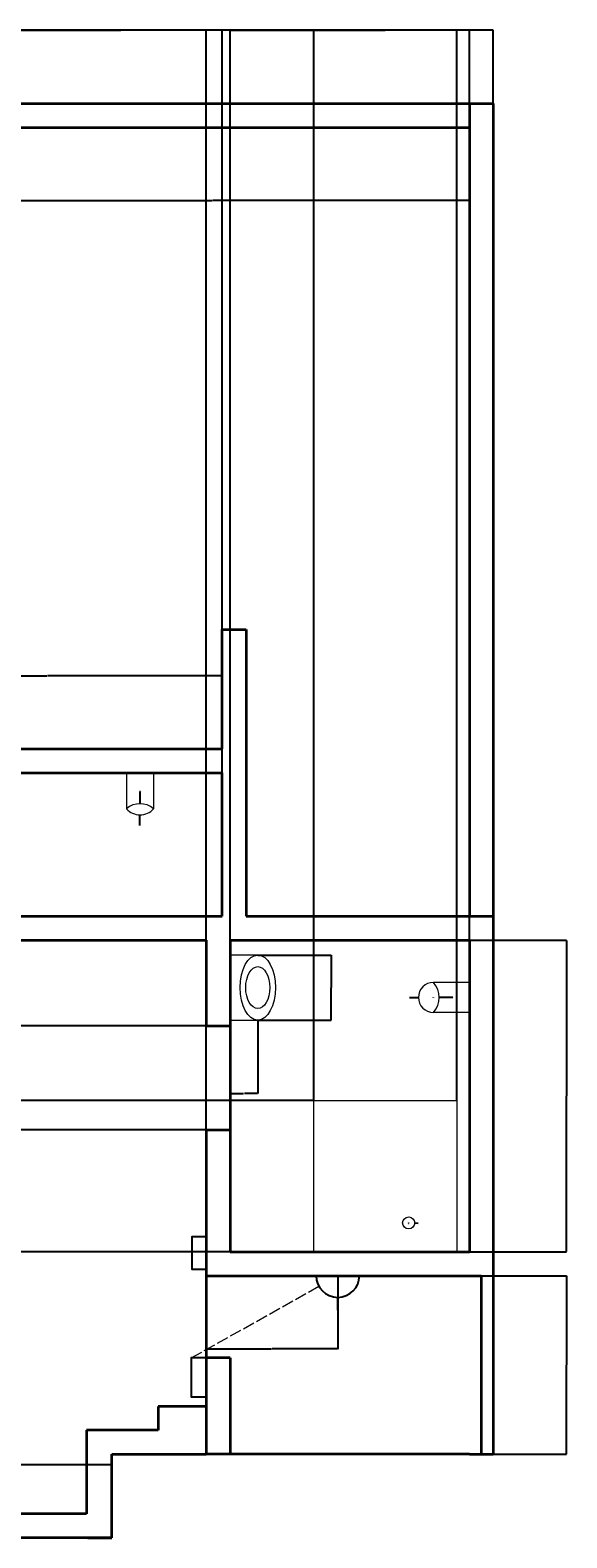
# Model space of a CAD drawing. Units: inches. Extents: x 2034 to 3646, y 962 to 2549.
# Tile 4 of 4: x 3108 to 3646, y 1036 to 2549. Entities that reach past the tile are written whole.
import ezdxf

# ---------------------------------------------------------------- set-up
doc = ezdxf.new("R2010")
doc.units = ezdxf.units.IN
doc.linetypes.add('ACAD_ISO02W100', pattern=[15, 12, -3])
for name, color, linetype, lineweight in [('A-ANNO-DIMS', 2, 'Continuous', 18), ('A-FLOR-FIXT', 9, 'Continuous', 18), ('E-LITE-CTRL', 7, 'Continuous', 25), ('E-POWR-DEVC', 7, 'Continuous', 25)]:
    doc.layers.add(name, color=color, linetype=linetype, lineweight=lineweight)
doc.layers.add('A-WALL', color=203, linetype='Continuous', lineweight=35, true_color=0xa780c2)
doc.layers.add('E-LITE-WIRE', color=103, linetype='ACAD_ISO02W100', lineweight=18, true_color=0x6dc08b)
doc.styles.get("Standard").update_dxf_attribs({"font": 'arial.ttf'})
doc.dimstyles.get("Standard").update_dxf_attribs({"dimtxt": 0.18, "dimasz": 0.18, "dimexe": 0.18, "dimexo": 0.0625, "dimgap": 0.09, "dimtad": 0, "dimtih": 1, "dimtoh": 1, "dimdec": 4, "dimzin": 0, "dimdsep": 46, "dimtxsty": 'Standard', "dimcen": 0.09, "dimadec": 0, "dimazin": 0, "dimtfac": 1, "dimtdec": 4, "dimtofl": 0, "dimtmove": 0, "dimatfit": 3, "dimfxl": 1, "dimtolj": 1, "dimtzin": 0, "dimarcsym": 0})

# ---------------------------------------------------------------- blocks, each defined once
blk = doc.blocks.new('*D4')
at = {"layer": 'A-ANNO-DIMS', "color": 0, "lineweight": -2, "transparency": 16777216}
for p, q in [((2108.2, 2475.7), (2108.2, 2549.3)), ((2108.4, 2549.1), (2839.8, 2549.1)), ((3572, 2549.1), (2840.5, 2549.1)), ((3572.2, 2475.7), (3572.2, 2549.3))]:
    blk.add_line(p, q, dxfattribs=at)
at = {"layer": 'A-ANNO-DIMS', "color": 0, "transparency": 16777216}
for points in [[(2108.4, 2549.1), (2108.4, 2549.1), (2108.2, 2549.1)], [(3572, 2549.1), (3572, 2549.1), (3572.2, 2549.1)]]:
    blk.add_solid(points, dxfattribs=at)
at = {"layer": 'Defpoints', "color": 0, "transparency": 16777216}
for p in [(3572.2, 2549.1), (2108.2, 2475.6), (3572.2, 2475.6)]:
    blk.add_point(p, dxfattribs=at)
at = {"layer": 'A-ANNO-DIMS', "color": 0, "transparency": 16777216, "insert": (2840.2, 2549.1), "char_height": 0.18, "attachment_point": 5}
blk.add_mtext('\\A1;1464', dxfattribs=at)
blk = doc.blocks.new('*D8')
at = {"layer": 'A-ANNO-DIMS', "color": 0, "lineweight": -2, "transparency": 16777216}
for p, q in [((2682.3, 1035.7), (2682.3, 1109.3)), ((2682.5, 1109.1), (2935.5, 1109.1)), ((3189.4, 1109.1), (2936.3, 1109.1)), ((3189.6, 1035.7), (3189.6, 1109.3))]:
    blk.add_line(p, q, dxfattribs=at)
at = {"layer": 'A-ANNO-DIMS', "color": 0, "transparency": 16777216}
for points in [[(2682.5, 1109.1), (2682.5, 1109.1), (2682.3, 1109.1)], [(3189.4, 1109.1), (3189.4, 1109.1), (3189.6, 1109.1)]]:
    blk.add_solid(points, dxfattribs=at)
at = {"layer": 'Defpoints', "color": 0, "transparency": 16777216}
for p in [(3189.6, 1109.1), (2682.3, 1035.6), (3189.6, 1035.6)]:
    blk.add_point(p, dxfattribs=at)
at = {"layer": 'A-ANNO-DIMS', "color": 0, "transparency": 16777216, "insert": (2935.9, 1109.1), "char_height": 0.18, "attachment_point": 5}
blk.add_mtext('\\A1;507.2', dxfattribs=at)
blk = doc.blocks.new('*D11')
at = {"layer": 'A-ANNO-DIMS', "color": 0, "lineweight": -2, "transparency": 16777216}
for p, q in [((3033.1, 2451.6), (3033.1, 2378)), ((3548.2, 2451.6), (3548.2, 2378)), ((3033.3, 2378.2), (3290.3, 2378.2)), ((3548, 2378.2), (3291, 2378.2))]:
    blk.add_line(p, q, dxfattribs=at)
at = {"layer": 'A-ANNO-DIMS', "color": 0, "transparency": 16777216}
for points in [[(3033.3, 2378.2), (3033.3, 2378.2), (3033.1, 2378.2)], [(3548, 2378.2), (3548, 2378.2), (3548.2, 2378.2)]]:
    blk.add_solid(points, dxfattribs=at)
at = {"layer": 'Defpoints', "color": 0, "transparency": 16777216}
for p in [(3033.1, 2451.6), (3548.2, 2451.6), (3033.1, 2378.2)]:
    blk.add_point(p, dxfattribs=at)
at = {"layer": 'A-ANNO-DIMS', "color": 0, "transparency": 16777216, "insert": (3290.7, 2378.2), "char_height": 0.18, "attachment_point": 5}
blk.add_mtext('\\A1;515.1', dxfattribs=at)
blk = doc.blocks.new('*D16')
at = {"layer": 'A-ANNO-DIMS', "color": 0, "lineweight": -2, "transparency": 16777216}
for p, q in [((2588.2, 1635.7), (2588.2, 2549.3)), ((2588.4, 2549.1), (2935.9, 2549.1)), ((3284, 2549.1), (2936.5, 2549.1)), ((3284.2, 1635.7), (3284.2, 2549.3))]:
    blk.add_line(p, q, dxfattribs=at)
at = {"layer": 'A-ANNO-DIMS', "color": 0, "transparency": 16777216}
for points in [[(2588.4, 2549.1), (2588.4, 2549.1), (2588.2, 2549.1)], [(3284, 2549.1), (3284, 2549.1), (3284.2, 2549.1)]]:
    blk.add_solid(points, dxfattribs=at)
at = {"layer": 'Defpoints', "color": 0, "transparency": 16777216}
for p in [(3284.2, 2549.1), (2588.2, 1635.6), (3284.2, 1635.6)]:
    blk.add_point(p, dxfattribs=at)
at = {"layer": 'A-ANNO-DIMS', "color": 0, "transparency": 16777216, "insert": (2936.2, 2549.1), "char_height": 0.18, "attachment_point": 5}
blk.add_mtext('\\A1;696', dxfattribs=at)
blk = doc.blocks.new('*D18')
at = {"layer": 'A-ANNO-DIMS', "color": 0, "lineweight": -2, "transparency": 16777216}
for p, q in [((3308.2, 1635.7), (3308.2, 2549.3)), ((3308.4, 2549.1), (3427.9, 2549.1)), ((3548, 2549.1), (3428.5, 2549.1)), ((3548.2, 1635.7), (3548.2, 2549.3))]:
    blk.add_line(p, q, dxfattribs=at)
at = {"layer": 'A-ANNO-DIMS', "color": 0, "transparency": 16777216}
for points in [[(3308.4, 2549.1), (3308.4, 2549.1), (3308.2, 2549.1)], [(3548, 2549.1), (3548, 2549.1), (3548.2, 2549.1)]]:
    blk.add_solid(points, dxfattribs=at)
at = {"layer": 'Defpoints', "color": 0, "transparency": 16777216}
for p in [(3548.2, 2549.1), (3308.2, 1635.6), (3548.2, 1635.6)]:
    blk.add_point(p, dxfattribs=at)
at = {"layer": 'A-ANNO-DIMS', "color": 0, "transparency": 16777216, "insert": (3428.2, 2549.1), "char_height": 0.18, "attachment_point": 5}
blk.add_mtext('\\A1;240', dxfattribs=at)
blk = doc.blocks.new('*D19')
at = {"layer": 'A-ANNO-DIMS', "color": 0, "lineweight": -2, "transparency": 16777216}
for p, q in [((3548.3, 1635.6), (3645.8, 1635.6)), ((3645.6, 1635.5), (3645.6, 1479.4)), ((3645.6, 1323), (3645.6, 1479.1)), ((3548.3, 1322.8), (3645.8, 1322.8))]:
    blk.add_line(p, q, dxfattribs=at)
at = {"layer": 'A-ANNO-DIMS', "color": 0, "transparency": 16777216}
for points in [[(3645.6, 1635.5), (3645.7, 1635.5), (3645.6, 1635.6)], [(3645.6, 1323), (3645.7, 1323), (3645.6, 1322.8)]]:
    blk.add_solid(points, dxfattribs=at)
at = {"layer": 'Defpoints', "color": 0, "transparency": 16777216}
for p in [(3548.2, 1635.6), (3645.6, 1635.6), (3548.2, 1322.8)]:
    blk.add_point(p, dxfattribs=at)
at = {"layer": 'A-ANNO-DIMS', "color": 0, "transparency": 16777216, "insert": (3645.6, 1479.2), "char_height": 0.18, "attachment_point": 5}
blk.add_mtext('\\A1;312.8', dxfattribs=at)
blk = doc.blocks.new('*D20')
at = {"layer": 'A-ANNO-DIMS', "color": 0, "lineweight": -2, "transparency": 16777216}
for p, q in [((3300.3, 1803.6), (2034.6, 1803.6)), ((2034.7, 1803.5), (2034.7, 1731.8)), ((2034.7, 1659.8), (2034.7, 1731.5)), ((3300.3, 1659.6), (2034.6, 1659.6))]:
    blk.add_line(p, q, dxfattribs=at)
at = {"layer": 'A-ANNO-DIMS', "color": 0, "transparency": 16777216}
for points in [[(2034.7, 1803.5), (2034.8, 1803.5), (2034.7, 1803.6)], [(2034.7, 1659.8), (2034.8, 1659.8), (2034.7, 1659.6)]]:
    blk.add_solid(points, dxfattribs=at)
at = {"layer": 'Defpoints', "color": 0, "transparency": 16777216}
for p in [(2034.7, 1803.6), (3300.3, 1803.6), (3300.3, 1659.6)]:
    blk.add_point(p, dxfattribs=at)
at = {"layer": 'A-ANNO-DIMS', "color": 0, "transparency": 16777216, "insert": (2034.7, 1731.6), "char_height": 0.18, "attachment_point": 5}
blk.add_mtext('\\A1;144', dxfattribs=at)
blk = doc.blocks.new('*D22')
at = {"layer": 'A-ANNO-DIMS', "color": 0, "lineweight": -2, "transparency": 16777216}
for p, q in [((3097.8, 1659.7), (3097.8, 2549.3)), ((3098, 2549.1), (3198.7, 2549.1)), ((3300.2, 2549.1), (3199.5, 2549.1)), ((3300.3, 1659.7), (3300.3, 2549.3))]:
    blk.add_line(p, q, dxfattribs=at)
at = {"layer": 'A-ANNO-DIMS', "color": 0, "transparency": 16777216}
for points in [[(3098, 2549.1), (3098, 2549.1), (3097.8, 2549.1)], [(3300.2, 2549.1), (3300.2, 2549.1), (3300.3, 2549.1)]]:
    blk.add_solid(points, dxfattribs=at)
at = {"layer": 'Defpoints', "color": 0, "transparency": 16777216}
for p in [(3300.3, 2549.1), (3097.8, 1659.6), (3300.3, 1659.6)]:
    blk.add_point(p, dxfattribs=at)
at = {"layer": 'A-ANNO-DIMS', "color": 0, "transparency": 16777216, "insert": (3199.1, 2549.1), "char_height": 0.18, "attachment_point": 5}
blk.add_mtext('\\A1;202.5', dxfattribs=at)
blk = doc.blocks.new('*D33')
at = {"layer": 'A-ANNO-DIMS', "color": 0, "lineweight": -2, "transparency": 16777216}
for p, q in [((2961.6, 1396.5), (2961.6, 2549.3)), ((2961.8, 2549.1), (3122.5, 2549.1)), ((3284, 2549.1), (3123.3, 2549.1)), ((3284.2, 1305), (3284.2, 2549.3))]:
    blk.add_line(p, q, dxfattribs=at)
at = {"layer": 'A-ANNO-DIMS', "color": 0, "transparency": 16777216}
for points in [[(2961.8, 2549.1), (2961.8, 2549.1), (2961.6, 2549.1)], [(3284, 2549.1), (3284, 2549.1), (3284.2, 2549.1)]]:
    blk.add_solid(points, dxfattribs=at)
at = {"layer": 'Defpoints', "color": 0, "transparency": 16777216}
for p in [(3284.2, 2549.1), (2961.6, 1396.4), (3284.2, 1304.9)]:
    blk.add_point(p, dxfattribs=at)
at = {"layer": 'A-ANNO-DIMS', "color": 0, "transparency": 16777216, "insert": (3122.9, 2549.1), "char_height": 0.18, "attachment_point": 5}
blk.add_mtext('\\A1;322.6', dxfattribs=at)
blk = doc.blocks.new('*D48')
at = {"layer": 'A-ANNO-DIMS', "color": 0, "lineweight": -2, "transparency": 16777216}
for p, q in [((3392.3, 1474.6), (3392.3, 2549.3)), ((3392.5, 2549.1), (3463.7, 2549.1)), ((3535.6, 2549.1), (3464.4, 2549.1)), ((3535.7, 1474.6), (3535.7, 2549.3))]:
    blk.add_line(p, q, dxfattribs=at)
at = {"layer": 'A-ANNO-DIMS', "color": 0, "transparency": 16777216}
for points in [[(3392.5, 2549.1), (3392.5, 2549.1), (3392.3, 2549.1)], [(3535.6, 2549.1), (3535.6, 2549.1), (3535.7, 2549.1)]]:
    blk.add_solid(points, dxfattribs=at)
at = {"layer": 'Defpoints', "color": 0, "transparency": 16777216}
for p in [(3535.7, 2549.1), (3392.3, 1474.6), (3535.7, 1474.6)]:
    blk.add_point(p, dxfattribs=at)
at = {"layer": 'A-ANNO-DIMS', "color": 0, "transparency": 16777216, "insert": (3464, 2549.1), "char_height": 0.18, "attachment_point": 5}
blk.add_mtext('\\A1;143.4', dxfattribs=at)
blk = doc.blocks.new('*D49')
at = {"layer": 'A-ANNO-DIMS', "color": 0, "lineweight": -2, "transparency": 16777216}
for p, q in [((3392.3, 1474.6), (2034.6, 1474.6)), ((2034.7, 1474.4), (2034.7, 1398.9)), ((2034.7, 1323), (2034.7, 1398.5)), ((3392.3, 1322.8), (2034.6, 1322.8))]:
    blk.add_line(p, q, dxfattribs=at)
at = {"layer": 'A-ANNO-DIMS', "color": 0, "transparency": 16777216}
for points in [[(2034.7, 1474.4), (2034.8, 1474.4), (2034.7, 1474.6)], [(2034.7, 1323), (2034.8, 1323), (2034.7, 1322.8)]]:
    blk.add_solid(points, dxfattribs=at)
at = {"layer": 'Defpoints', "color": 0, "transparency": 16777216}
for p in [(2034.7, 1474.6), (3392.3, 1474.6), (3392.3, 1322.8)]:
    blk.add_point(p, dxfattribs=at)
at = {"layer": 'A-ANNO-DIMS', "color": 0, "transparency": 16777216, "insert": (2034.7, 1398.7), "char_height": 0.18, "attachment_point": 5}
blk.add_mtext('\\A1;151.76', dxfattribs=at)
blk = doc.blocks.new('*D51')
at = {"layer": 'A-ANNO-DIMS', "color": 0, "lineweight": -2, "transparency": 16777216}
for p, q in [((2949.1, 1827.7), (2949.1, 1901.3)), ((2949.3, 1901.1), (3124.3, 1901.1)), ((3300.2, 1901.1), (3125.1, 1901.1)), ((3300.3, 1827.7), (3300.3, 1901.3))]:
    blk.add_line(p, q, dxfattribs=at)
at = {"layer": 'A-ANNO-DIMS', "color": 0, "transparency": 16777216}
for points in [[(2949.3, 1901.1), (2949.3, 1901.1), (2949.1, 1901.1)], [(3300.2, 1901.1), (3300.2, 1901.1), (3300.3, 1901.1)]]:
    blk.add_solid(points, dxfattribs=at)
at = {"layer": 'Defpoints', "color": 0, "transparency": 16777216}
for p in [(3300.3, 1901.1), (2949.1, 1827.6), (3300.3, 1827.6)]:
    blk.add_point(p, dxfattribs=at)
at = {"layer": 'A-ANNO-DIMS', "color": 0, "transparency": 16777216, "insert": (3124.7, 1901.1), "char_height": 0.18, "attachment_point": 5}
blk.add_mtext('\\A1;351.2', dxfattribs=at)
blk = doc.blocks.new('*D52')
at = {"layer": 'A-ANNO-DIMS', "color": 0, "lineweight": -2, "transparency": 16777216}
for p, q in [((3284.1, 1549.7), (2034.6, 1549.7)), ((2034.7, 1549.5), (2034.7, 1497.7)), ((2034.7, 1445.5), (2034.7, 1497.3)), ((3284.1, 1445.3), (2034.6, 1445.3))]:
    blk.add_line(p, q, dxfattribs=at)
at = {"layer": 'A-ANNO-DIMS', "color": 0, "transparency": 16777216}
for points in [[(2034.7, 1549.5), (2034.8, 1549.5), (2034.7, 1549.7)], [(2034.7, 1445.5), (2034.8, 1445.5), (2034.7, 1445.3)]]:
    blk.add_solid(points, dxfattribs=at)
at = {"layer": 'Defpoints', "color": 0, "transparency": 16777216}
for p in [(2034.7, 1549.7), (3284.2, 1549.7), (3284.2, 1445.3)]:
    blk.add_point(p, dxfattribs=at)
at = {"layer": 'A-ANNO-DIMS', "color": 0, "transparency": 16777216, "insert": (2034.7, 1497.5), "char_height": 0.18, "attachment_point": 5}
blk.add_mtext('\\A1;104.39', dxfattribs=at)
blk = doc.blocks.new('*D53')
at = {"layer": 'A-ANNO-DIMS', "color": 0, "lineweight": -2, "transparency": 16777216}
for p, q in [((3560.3, 1298.8), (3645.8, 1298.8)), ((3645.6, 1298.6), (3645.6, 1209.4)), ((3645.6, 1119.8), (3645.6, 1209.1)), ((3560.3, 1119.6), (3645.8, 1119.6))]:
    blk.add_line(p, q, dxfattribs=at)
at = {"layer": 'A-ANNO-DIMS', "color": 0, "transparency": 16777216}
for points in [[(3645.6, 1298.6), (3645.7, 1298.6), (3645.6, 1298.8)], [(3645.6, 1119.8), (3645.7, 1119.8), (3645.6, 1119.6)]]:
    blk.add_solid(points, dxfattribs=at)
at = {"layer": 'Defpoints', "color": 0, "transparency": 16777216}
for p in [(3560.2, 1298.8), (3645.6, 1298.8), (3560.2, 1119.6)]:
    blk.add_point(p, dxfattribs=at)
at = {"layer": 'A-ANNO-DIMS', "color": 0, "transparency": 16777216, "insert": (3645.6, 1209.2), "char_height": 0.18, "attachment_point": 5}
blk.add_mtext('\\A1;179.2', dxfattribs=at)
blk = doc.blocks.new('*D59')
at = {"layer": 'A-ANNO-DIMS', "color": 0, "lineweight": -2, "transparency": 16777216}
for p, q in [((3284.2, 1298.8), (3284.2, 1225.2)), ((3416.2, 1298.8), (3416.2, 1225.2)), ((3284.4, 1225.4), (3349.9, 1225.4)), ((3416, 1225.4), (3350.5, 1225.4))]:
    blk.add_line(p, q, dxfattribs=at)
at = {"layer": 'A-ANNO-DIMS', "color": 0, "transparency": 16777216}
for points in [[(3284.4, 1225.4), (3284.4, 1225.3), (3284.2, 1225.4)], [(3416, 1225.4), (3416, 1225.3), (3416.2, 1225.4)]]:
    blk.add_solid(points, dxfattribs=at)
at = {"layer": 'Defpoints', "color": 0, "transparency": 16777216}
for p in [(3284.2, 1298.8), (3416.2, 1298.8), (3284.2, 1225.4)]:
    blk.add_point(p, dxfattribs=at)
at = {"layer": 'A-ANNO-DIMS', "color": 0, "transparency": 16777216, "insert": (3350.2, 1225.4), "char_height": 0.18, "attachment_point": 5}
blk.add_mtext('\\A1;132', dxfattribs=at)
blk = doc.blocks.new('*D61')
at = {"layer": 'A-ANNO-DIMS', "color": 0, "lineweight": -2, "transparency": 16777216}
for p, q in [((3336.1, 1620.7), (3409.7, 1620.7)), ((3409.5, 1620.6), (3409.5, 1588.2)), ((3409.5, 1555.5), (3409.5, 1587.9)), ((3336.1, 1555.3), (3409.7, 1555.3))]:
    blk.add_line(p, q, dxfattribs=at)
at = {"layer": 'A-ANNO-DIMS', "color": 0, "transparency": 16777216}
for points in [[(3409.5, 1620.6), (3409.5, 1620.6), (3409.5, 1620.7)], [(3409.5, 1555.5), (3409.5, 1555.5), (3409.5, 1555.3)]]:
    blk.add_solid(points, dxfattribs=at)
at = {"layer": 'Defpoints', "color": 0, "transparency": 16777216}
for p in [(3336, 1620.7), (3336, 1555.3), (3409.5, 1555.3)]:
    blk.add_point(p, dxfattribs=at)
at = {"layer": 'A-ANNO-DIMS', "color": 0, "transparency": 16777216, "insert": (3409.5, 1588), "char_height": 0.18, "attachment_point": 5}
blk.add_mtext('\\A1;65.41', dxfattribs=at)
blk = doc.blocks.new('*D62')
at = {"layer": 'A-ANNO-DIMS', "color": 0, "lineweight": -2, "transparency": 16777216}
for p, q in [((3308.2, 1555.3), (3308.2, 1481.7)), ((3336, 1555.3), (3336, 1481.7)), ((3308.4, 1481.9), (3321.7, 1481.9)), ((3335.9, 1481.9), (3322.6, 1481.9))]:
    blk.add_line(p, q, dxfattribs=at)
at = {"layer": 'A-ANNO-DIMS', "color": 0, "transparency": 16777216}
for points in [[(3308.4, 1481.9), (3308.4, 1481.9), (3308.2, 1481.9)], [(3335.9, 1481.9), (3335.9, 1481.9), (3336, 1481.9)]]:
    blk.add_solid(points, dxfattribs=at)
at = {"layer": 'Defpoints', "color": 0, "transparency": 16777216}
for p in [(3308.2, 1555.3), (3336, 1555.3), (3308.2, 1481.9)]:
    blk.add_point(p, dxfattribs=at)
at = {"layer": 'A-ANNO-DIMS', "color": 0, "transparency": 16777216, "insert": (3322.1, 1481.9), "char_height": 0.18, "attachment_point": 5}
blk.add_mtext('\\A1;27.844', dxfattribs=at)
blk = doc.blocks.new('*D68')
at = {"layer": 'A-ANNO-DIMS', "color": 0, "lineweight": -2, "transparency": 16777216}
for p, q in [((3495.1, 1578.2), (3495.3, 1578.2)), ((3495.2, 1578.1), (3495.2, 1578.3)), ((3531.5, 1578.2), (3518.1, 1578.2))]:
    blk.add_line(p, q, dxfattribs=at)
at = {"layer": 'A-ANNO-DIMS', "color": 0, "transparency": 16777216}
blk.add_solid([(3518.1, 1578.2), (3518.1, 1578.1), (3517.9, 1578.2)], dxfattribs=at)
at = {"layer": 'Defpoints', "color": 0, "transparency": 16777216}
for p in [(3495.2, 1578.2), (3517.9, 1578.2)]:
    blk.add_point(p, dxfattribs=at)
at = {"layer": 'A-ANNO-DIMS', "color": 0, "transparency": 16777216, "insert": (3532.1, 1578.2), "char_height": 0.18, "attachment_point": 5}
blk.add_mtext('\\A1;R22.707', dxfattribs=at)
blk = doc.blocks.new('*D69')
at = {"layer": 'A-ANNO-DIMS', "color": 0, "lineweight": -2, "transparency": 16777216}
for p, q in [((3416.1, 1298.8), (3416.3, 1298.8)), ((3416.2, 1298.7), (3416.2, 1298.9)), ((3416.2, 1264.1), (3416.2, 1276.9)), ((3416.4, 1264.1), (3416.2, 1264.1))]:
    blk.add_line(p, q, dxfattribs=at)
at = {"layer": 'A-ANNO-DIMS', "color": 0, "transparency": 16777216}
blk.add_solid([(3416.2, 1276.9), (3416.2, 1276.9), (3416.2, 1277.1)], dxfattribs=at)
at = {"layer": 'Defpoints', "color": 0, "transparency": 16777216}
for p in [(3416.2, 1298.8), (3416.2, 1277.1)]:
    blk.add_point(p, dxfattribs=at)
at = {"layer": 'A-ANNO-DIMS', "color": 0, "transparency": 16777216, "insert": (3416.9, 1264.1), "char_height": 0.18, "attachment_point": 5}
blk.add_mtext('\\A1;R21.733', dxfattribs=at)
blk = doc.blocks.new('*D71')
at = {"layer": 'A-ANNO-DIMS', "color": 0, "lineweight": -2, "transparency": 16777216}
for p, q in [((3218.1, 1785), (3217.9, 1785)), ((3217.9, 1785), (3217.9, 1772.8)), ((3217.9, 1751.8), (3217.9, 1752)), ((3217.9, 1751.9), (3218, 1751.9))]:
    blk.add_line(p, q, dxfattribs=at)
at = {"layer": 'A-ANNO-DIMS', "color": 0, "transparency": 16777216}
blk.add_solid([(3217.9, 1772.8), (3218, 1772.8), (3217.9, 1772.6)], dxfattribs=at)
at = {"layer": 'Defpoints', "color": 0, "transparency": 16777216}
for p in [(3217.9, 1772.6), (3217.9, 1751.9)]:
    blk.add_point(p, dxfattribs=at)
at = {"layer": 'A-ANNO-DIMS', "color": 0, "transparency": 16777216, "insert": (3218.7, 1785), "char_height": 0.18, "attachment_point": 5}
blk.add_mtext('\\A1;R20.705', dxfattribs=at)
blk = doc.blocks.new('*D74')
at = {"layer": 'A-ANNO-DIMS', "color": 0, "lineweight": -2, "transparency": 16777216}
for p, q in [((3217.9, 1779.1), (3217.9, 1779.3)), ((3217.9, 1779.2), (3218, 1779.2)), ((3217.9, 1750.8), (3217.9, 1761.3)), ((3217.8, 1750.8), (3217.9, 1750.8))]:
    blk.add_line(p, q, dxfattribs=at)
at = {"layer": 'A-ANNO-DIMS', "color": 0, "transparency": 16777216}
blk.add_solid([(3217.9, 1761.3), (3218, 1761.3), (3217.9, 1761.4)], dxfattribs=at)
at = {"layer": 'Defpoints', "color": 0, "transparency": 16777216}
for p in [(3217.9, 1779.2), (3217.9, 1761.4)]:
    blk.add_point(p, dxfattribs=at)
at = {"layer": 'A-ANNO-DIMS', "color": 0, "transparency": 16777216, "insert": (3217.2, 1750.8), "char_height": 0.18, "attachment_point": 5}
blk.add_mtext('\\A1;R17.743', dxfattribs=at)
blk = doc.blocks.new('*D75')
at = {"layer": 'A-ANNO-DIMS', "color": 0, "lineweight": -2, "transparency": 16777216}
for p, q in [((3488.1, 1578.2), (3497, 1578.2)), ((3512.1, 1578.2), (3512.3, 1578.2)), ((3512.2, 1578.1), (3512.2, 1578.3))]:
    blk.add_line(p, q, dxfattribs=at)
at = {"layer": 'A-ANNO-DIMS', "color": 0, "transparency": 16777216}
blk.add_solid([(3497, 1578.2), (3497, 1578.1), (3497.1, 1578.2)], dxfattribs=at)
at = {"layer": 'Defpoints', "color": 0, "transparency": 16777216}
for p in [(3497.1, 1578.2), (3512.2, 1578.2)]:
    blk.add_point(p, dxfattribs=at)
at = {"layer": 'A-ANNO-DIMS', "color": 0, "transparency": 16777216, "insert": (3487.6, 1578.2), "char_height": 0.18, "attachment_point": 5}
blk.add_mtext('\\A1;R15.06', dxfattribs=at)
blk = doc.blocks.new('*D79')
at = {"layer": 'A-ANNO-DIMS', "color": 0, "lineweight": -2, "transparency": 16777216}
for p, q in [((3487.3, 1351.7), (3487.4, 1351.7)), ((3487.4, 1351.7), (3487.4, 1351.8)), ((3497, 1351.1), (3493.6, 1351.4))]:
    blk.add_line(p, q, dxfattribs=at)
at = {"layer": 'A-ANNO-DIMS', "color": 0, "transparency": 16777216}
blk.add_solid([(3493.6, 1351.4), (3493.5, 1351.3), (3493.4, 1351.4)], dxfattribs=at)
at = {"layer": 'Defpoints', "color": 0, "transparency": 16777216}
for p in [(3481.3, 1352.1), (3493.4, 1351.4)]:
    blk.add_point(p, dxfattribs=at)
at = {"layer": 'A-ANNO-DIMS', "color": 0, "transparency": 16777216, "insert": (3497.5, 1351.1), "char_height": 0.18, "attachment_point": 5}
blk.add_mtext('\\A1;∅12.06', dxfattribs=at)

msp = doc.modelspace()

# ---------------------------------------------------------------- linework, layer by layer
at = {"layer": 'A-FLOR-FIXT'}
for p, q in [((3204.4683, 1803.6388), (3204.4683, 1767.6388)), ((3231.4136, 1803.6388), (3231.4136, 1767.6388)), ((3336.0415, 1620.7492), (3308.1976, 1620.7492)), ((3308.1976, 1620.7492), (3308.1976, 1555.3406)), ((3548.1976, 1593.2385), (3512.1976, 1593.2385)), ((3548.1976, 1563.1193), (3512.1976, 1563.1193)), ((3308.1976, 1555.3406), (3336.0415, 1555.3406))]:
    msp.add_line(p, q, dxfattribs=at)
msp.add_lwpolyline([(3535.7476, 1322.8257), (3392.3387, 1322.8257), (3392.3387, 1474.5871), (3535.7476, 1474.5871)], close=True, dxfattribs=at)
msp.add_circle((3487.354, 1351.7404), 6.0298, dxfattribs=at)
for centre, radius, start, end in [((3217.941, 1751.917), 20.7048, 49.4054444, 130.5945556), ((3217.941, 1779.184), 17.7427, 220.5945556, 319.4054444), ((3512.1976, 1578.1789), 15.0596, 90, 270), ((3495.2031, 1578.1789), 22.7069, 318.4543472, 41.5456528)]:
    msp.add_arc(centre, radius, start, end, dxfattribs=at)
for major_axis, ratio in [((0, -32.7043), 0.543307181), ((0, -21.1161), 0.573171594)]:
    msp.add_ellipse((3336.0415, 1588.0449), major_axis=major_axis, ratio=ratio, dxfattribs=at)
at = {"layer": 'A-WALL'}
for p, q in [((3308.1976, 2475.6388), (3548.1976, 2475.6388)), ((3548.1976, 2475.6388), (3548.1976, 1659.6388)), ((3548.1976, 2475.6388), (3572.1976, 2475.6388)), ((3572.1976, 2475.6388), (3572.1976, 1119.6388)), ((3033.1244, 2451.6388), (3284.1976, 2451.6388)), ((3284.1976, 2451.6388), (3548.1976, 2451.6388)), ((3300.3398, 1947.6388), (3324.3398, 1947.6388)), ((3300.3398, 1827.6388), (3300.3398, 1947.6388)), ((3324.3398, 1947.6388), (3324.3398, 1659.6388)), ((2949.1244, 1827.6388), (3300.3398, 1827.6388)), ((2826.4216, 1803.6388), (3300.3398, 1803.6388)), ((3300.3398, 1659.6388), (3300.3398, 1803.6388)), ((2729.8258, 1659.6388), (3300.3398, 1659.6388)), ((3324.3398, 1659.6388), (3548.1976, 1659.6388)), ((3548.1976, 1659.6388), (3572.1976, 1659.6388)), ((2588.1976, 1635.6388), (3284.1976, 1635.6388)), ((3284.1976, 1635.6388), (3284.1976, 1549.6921)), ((3308.1976, 1635.6388), (3308.1976, 1445.3057)), ((3308.1976, 1635.6388), (3548.1976, 1635.6388)), ((3548.1976, 1635.6388), (3548.1976, 1322.8257)), ((3284.1976, 1549.6921), (3308.1976, 1549.6921)), ((3284.1976, 1445.3057), (3308.1976, 1445.3057)), ((3284.1976, 1445.3057), (3284.1976, 1119.6388)), ((3308.1976, 1445.3057), (3308.1976, 1322.8257)), ((3308.1976, 1322.8257), (3548.1976, 1322.8257)), ((3284.1976, 1298.8257), (3548.1976, 1298.8257)), ((3548.1976, 1298.8257), (3560.1976, 1298.8257)), ((3560.1976, 1298.8257), (3560.1976, 1119.6388)), ((3308.1976, 1216.2228), (3284.1976, 1216.2228)), ((3308.1976, 1216.2228), (3308.1976, 1119.6388)), ((3284.1976, 1167.6388), (3236.1976, 1167.6388)), ((3236.1976, 1167.6388), (3236.1976, 1143.6388)), ((3236.1976, 1143.6388), (3164.1976, 1143.6388)), ((3164.1976, 1143.6388), (3164.1976, 1059.6388)), ((3189.5638, 1035.6388), (3189.5638, 1119.6388)), ((3189.5638, 1119.6388), (3284.1976, 1119.6388)), ((3548.1976, 1119.6388), (3284.1976, 1119.6388)), ((3548.1976, 1119.6388), (3572.1976, 1119.6388)), ((3164.1976, 1059.6388), (2708.1976, 1059.6388)), ((3189.5638, 1035.6388), (2682.3208, 1035.6388)), ((3165.5638, 1035.6388), (3189.5638, 1035.6388))]:
    msp.add_line(p, q, dxfattribs=at)
msp.add_lwpolyline([(2108.1976, 1407.6388), (2108.1976, 2475.6388), (3308.1976, 2475.6388)], dxfattribs=at)
at = {"layer": 'E-LITE-CTRL'}
msp.add_lwpolyline([(3284.1976, 1216.2228), (3269.3292, 1216.2228), (3269.3292, 1177.0911), (3284.1976, 1177.0911)], close=True, dxfattribs=at)
at = {"layer": 'E-LITE-WIRE'}
msp.add_line((3269.3292, 1216.2228), (3397.2553, 1288.172), dxfattribs=at)
at = {"layer": 'E-POWR-DEVC'}
msp.add_lwpolyline([(3284.1976, 1304.9248), (3270.1214, 1304.9248), (3270.1214, 1338.1694), (3284.1976, 1338.1694)], close=True, dxfattribs=at)
msp.add_arc((3416.1976, 1298.8257), 21.7328, 180, 0, dxfattribs=at)

# ---------------------------------------------------------------- dimensions: what is measured, and where the dimension line sits
at = {"layer": 'A-ANNO-DIMS'}
for base, p1, p2, override, picture, middle in [((3572.1976, 2549.0888), (2108.1976, 2475.6388), (3572.1976, 2475.6388), {"dimdec": 0, "dimlfac": 1, "dimrnd": 0, "dimzin": 0, "dimdsep": 46, "dimlunit": 2}, '*D4', (2840.1976, 2549.0888)), ((3284.1976, 2549.0888), (2588.1976, 1635.6388), (3284.1976, 1635.6388), {"dimdec": 0, "dimlfac": 1, "dimrnd": 0, "dimzin": 0, "dimdsep": 46, "dimlunit": 2}, '*D16', (2936.1976, 2549.0888)), ((3284.1976, 2549.0888), (2961.5838, 1396.4302), (3284.1976, 1304.9248), {"dimdec": 1, "dimlfac": 1, "dimrnd": 0, "dimzin": 0, "dimdsep": 46, "dimlunit": 2}, '*D33', (3122.8907, 2549.0888)), ((3300.3398, 2549.0888), (3097.8265, 1659.6388), (3300.3398, 1659.6388), {"dimdec": 1, "dimlfac": 1, "dimrnd": 0, "dimzin": 0, "dimdsep": 46, "dimlunit": 2}, '*D22', (3199.0831, 2549.0888)), ((3548.1976, 2549.0888), (3308.1976, 1635.6388), (3548.1976, 1635.6388), {"dimdec": 0, "dimlfac": 1, "dimrnd": 0, "dimzin": 0, "dimdsep": 46, "dimlunit": 2}, '*D18', (3428.1976, 2549.0888)), ((3535.7476, 2549.0888), (3392.3387, 1474.5871), (3535.7476, 1474.5871), {"dimdec": 1, "dimlfac": 1, "dimrnd": 0, "dimzin": 0, "dimdsep": 46, "dimlunit": 2}, '*D48', (3464.0431, 2549.0888)), ((3300.3398, 1901.0888), (2949.1244, 1827.6388), (3300.3398, 1827.6388), {"dimdec": 1, "dimlfac": 1, "dimrnd": 0, "dimzin": 0, "dimdsep": 46, "dimlunit": 2}, '*D51', (3124.7321, 1901.0888)), ((3189.5638, 1109.0888), (2682.3208, 1035.6388), (3189.5638, 1035.6388), {"dimdec": 1, "dimlfac": 1, "dimrnd": 0, "dimzin": 0, "dimdsep": 46, "dimlunit": 2}, '*D8', (2935.9423, 1109.0888))]:
    dim = msp.add_linear_dim(base=base, p1=p1, p2=p2, dimstyle='Standard', override=override, dxfattribs=at)
    dim.commit()
    dim.dimension.update_dxf_attribs({"geometry": picture, "text_midpoint": middle})
for base, p1, p2, angle, override, picture, middle in [((3033.1244, 2378.1888), (3548.1976, 2451.6388), (3033.1244, 2451.6388), 180, {"dimdec": 1, "dimlfac": 1, "dimrnd": 0, "dimzin": 0, "dimdsep": 46, "dimlunit": 2}, '*D11', (3290.661, 2378.1888)), ((2034.7476, 1803.6388), (3300.3398, 1659.6388), (3300.3398, 1803.6388), 90, {"dimdec": 0, "dimlfac": 1, "dimrnd": 0, "dimzin": 0, "dimdsep": 46, "dimlunit": 2}, '*D20', (2034.7476, 1731.6388)), ((3645.6476, 1635.6388), (3548.1976, 1322.8257), (3548.1976, 1635.6388), 90, {"dimdec": 1, "dimlfac": 1, "dimrnd": 0, "dimzin": 0, "dimdsep": 46, "dimlunit": 2}, '*D19', (3645.6476, 1479.2323)), ((3409.4915, 1555.3406), (3336.0415, 1620.7492), (3336.0415, 1555.3406), 270, {"dimdec": 2, "dimlfac": 1, "dimrnd": 0, "dimzin": 0, "dimdsep": 46, "dimlunit": 2}, '*D61', (3409.4915, 1588.0449)), ((2034.7476, 1549.6921), (3284.1976, 1445.3057), (3284.1976, 1549.6921), 90, {"dimdec": 2, "dimlfac": 1, "dimrnd": 0, "dimzin": 0, "dimdsep": 46, "dimlunit": 2}, '*D52', (2034.7476, 1497.4989)), ((3308.1976, 1481.8906), (3336.0415, 1555.3406), (3308.1976, 1555.3406), 180, {"dimdec": 3, "dimlfac": 1, "dimrnd": 0, "dimzin": 0, "dimdsep": 46, "dimlunit": 2}, '*D62', (3322.1196, 1481.8906)), ((2034.7476, 1474.5871), (3392.3387, 1322.8257), (3392.3387, 1474.5871), 90, {"dimdec": 2, "dimlfac": 1, "dimrnd": 0, "dimzin": 0, "dimdsep": 46, "dimlunit": 2}, '*D49', (2034.7476, 1398.7064)), ((3284.1976, 1225.3757), (3416.1976, 1298.8257), (3284.1976, 1298.8257), 180, {"dimdec": 0, "dimlfac": 1, "dimrnd": 0, "dimzin": 0, "dimdsep": 46, "dimlunit": 2}, '*D59', (3350.1976, 1225.3757)), ((3645.6476, 1298.8257), (3560.1976, 1119.6388), (3560.1976, 1298.8257), 90, {"dimdec": 1, "dimlfac": 1, "dimrnd": 0, "dimzin": 0, "dimdsep": 46, "dimlunit": 2}, '*D53', (3645.6476, 1209.2323))]:
    dim = msp.add_linear_dim(base=base, p1=p1, p2=p2, angle=angle, dimstyle='Standard', override=override, dxfattribs=at)
    dim.commit()
    dim.dimension.update_dxf_attribs({"geometry": picture, "text_midpoint": middle})
for center, mpoint, override, picture, middle in [((3217.941, 1779.184), (3217.941, 1761.4413), {"dimdec": 3, "dimlfac": 1, "dimrnd": 0, "dimzin": 0, "dimdsep": 46, "dimlunit": 2}, '*D74', (3217.2112, 1750.7957)), ((3217.941, 1751.917), (3217.941, 1772.6218), {"dimdec": 3, "dimlfac": 1, "dimrnd": 0, "dimzin": 0, "dimdsep": 46, "dimlunit": 2}, '*D71', (3218.6714, 1785.0446)), ((3512.1976, 1578.1789), (3497.138, 1578.179), {"dimdec": 2, "dimlfac": 1, "dimrnd": 0, "dimzin": 0, "dimdsep": 46, "dimlunit": 2}, '*D75', (3488.1023, 1578.179)), ((3495.2031, 1578.1789), (3517.9101, 1578.179), {"dimdec": 3, "dimlfac": 1, "dimrnd": 0, "dimzin": 0, "dimdsep": 46, "dimlunit": 2}, '*D68', (3531.5342, 1578.179)), ((3416.1976, 1298.8257), (3416.198, 1277.0929), {"dimdec": 3, "dimlfac": 1, "dimrnd": 0, "dimzin": 0, "dimdsep": 46, "dimlunit": 2}, '*D69', (3416.928, 1264.0532))]:
    dim = msp.add_radius_dim(center=center, mpoint=mpoint, dimstyle='Standard', override=override, dxfattribs=at)
    dim.commit()
    dim.dimension.update_dxf_attribs({"geometry": picture, "text_midpoint": middle, "dimtype": 164})
dim = msp.add_diameter_dim_2p(p1=(3481.3359, 1352.1165), p2=(3493.372, 1351.3642), dimstyle='Standard', override={"dimdec": 2, "dimlfac": 1, "dimrnd": 0, "dimzin": 0, "dimdsep": 46, "dimlunit": 2}, dxfattribs=at)
dim.commit()
dim.dimension.update_dxf_attribs({"geometry": '*D79', "text_midpoint": (3496.9829, 1351.1386), "dimtype": 163})

doc.saveas('drawing.dxf')
